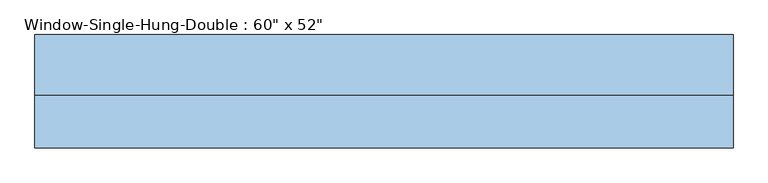
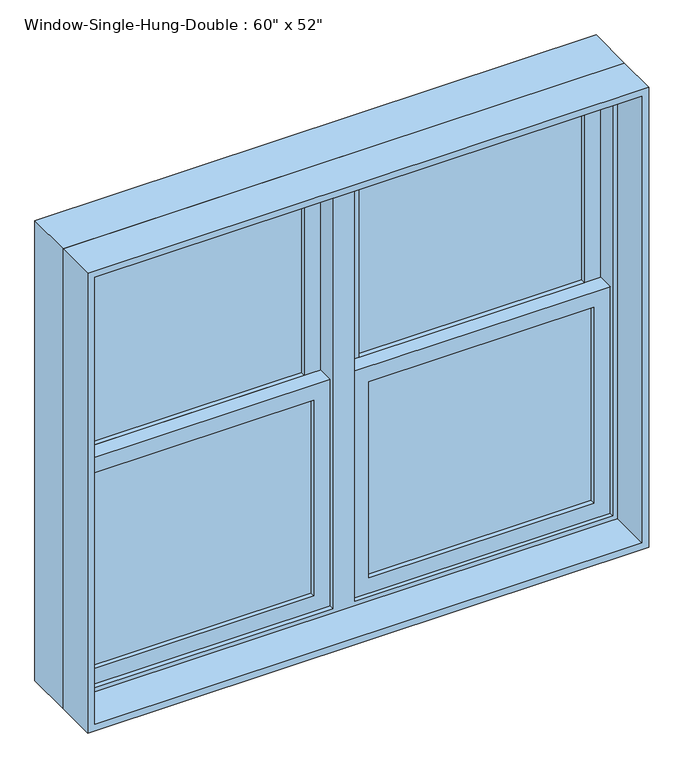
"""IFC4 building model written with IfcOpenShell, lengths in millimetres: window geometry."""

from ifc_helpers import new_model, si_unit, frame, origin, place, context, project, spatial, polyline, outline, extrude, source, transform, mapped, element, save


def window_bf3e2632(model_context):
    return source(origin(), model_context, "Body", "SweptSolid", [
        extrude(outline(polyline([(2235.2, 762.0), (2235.2, -762.0), (914.4, -762.0), (914.4, 762.0), (2235.2, 762.0)]), holes=[polyline([(2216.15, 742.95), (933.45, 742.95), (933.45, -742.95), (2216.15, -742.95), (2216.15, 742.95)])]), frame((0.0, -114.3, 0.0), z_axis=(0.0, 1.0, 0.0), x_axis=(0.0, 0.0, 1.0)), (0.0, 0.0, 1.0), 114.3),
        extrude(outline(polyline([(2203.45, 30.1625), (1552.575, 30.1625), (1552.575, 730.25), (2203.45, 730.25), (2203.45, 30.1625)]), holes=[polyline([(2159.0, 685.8), (1597.025, 685.8), (1597.025, 74.6125), (2159.0, 74.6125), (2159.0, 685.8)])]), frame((0.0, 57.15, 0.0), z_axis=(0.0, 1.0, 0.0), x_axis=(0.0, 0.0, 1.0)), (0.0, 0.0, 1.0), 44.45),
        extrude(outline(polyline([(1597.025, 30.1625), (946.15, 30.1625), (946.15, 730.25), (1597.025, 730.25), (1597.025, 30.1625)]), holes=[polyline([(1552.575, 685.8), (990.6, 685.8), (990.6, 74.6125), (1552.575, 74.6125), (1552.575, 685.8)])]), frame((0.0, 12.7, 0.0), z_axis=(0.0, 1.0, 0.0), x_axis=(0.0, 0.0, 1.0)), (0.0, 0.0, 1.0), 44.45),
        extrude(outline(polyline([(685.8, 88.9), (685.8, 82.55), (74.6125, 82.55), (74.6125, 88.9), (685.8, 88.9)])), frame((0.0, 0.0, 1597.025), z_axis=(0.0, 0.0, 1.0), x_axis=(1.0, 0.0, 0.0)), (0.0, 0.0, 1.0), 561.975),
        extrude(outline(polyline([(74.6125, 76.2), (685.8, 76.2), (685.8, 69.85), (74.6125, 69.85), (74.6125, 76.2)])), frame((0.0, 0.0, 1597.025), z_axis=(0.0, 0.0, 1.0), x_axis=(1.0, 0.0, 0.0)), (0.0, 0.0, 1.0), 561.975),
        extrude(outline(polyline([(685.8, 44.45), (685.8, 38.1), (74.6125, 38.1), (74.6125, 44.45), (685.8, 44.45)])), frame((0.0, 0.0, 990.6), z_axis=(0.0, 0.0, 1.0), x_axis=(1.0, 0.0, 0.0)), (0.0, 0.0, 1.0), 561.975),
        extrude(outline(polyline([(74.6125, 31.75), (685.8, 31.75), (685.8, 25.4), (74.6125, 25.4), (74.6125, 31.75)])), frame((0.0, 0.0, 990.6), z_axis=(0.0, 0.0, 1.0), x_axis=(1.0, 0.0, 0.0)), (0.0, 0.0, 1.0), 561.975),
        extrude(outline(polyline([(2203.45, -730.25), (1552.575, -730.25), (1552.575, -30.1625), (2203.45, -30.1625), (2203.45, -730.25)]), holes=[polyline([(2159.0, -74.6125), (1597.025, -74.6125), (1597.025, -685.8), (2159.0, -685.8), (2159.0, -74.6125)])]), frame((0.0, 57.15, 0.0), z_axis=(0.0, 1.0, 0.0), x_axis=(0.0, 0.0, 1.0)), (0.0, 0.0, 1.0), 44.45),
        extrude(outline(polyline([(1597.025, -730.25), (946.15, -730.25), (946.15, -30.1625), (1597.025, -30.1625), (1597.025, -730.25)]), holes=[polyline([(1552.575, -74.6125), (990.6, -74.6125), (990.6, -685.8), (1552.575, -685.8), (1552.575, -74.6125)])]), frame((0.0, 12.7, 0.0), z_axis=(0.0, 1.0, 0.0), x_axis=(0.0, 0.0, 1.0)), (0.0, 0.0, 1.0), 44.45),
        extrude(outline(polyline([(-685.8, 88.9), (-74.6125, 88.9), (-74.6125, 82.55), (-685.8, 82.55), (-685.8, 88.9)])), frame((0.0, 0.0, 1597.025), z_axis=(0.0, 0.0, 1.0), x_axis=(1.0, 0.0, 0.0)), (0.0, 0.0, 1.0), 561.975),
        extrude(outline(polyline([(-74.6125, 76.2), (-74.6125, 69.85), (-685.8, 69.85), (-685.8, 76.2), (-74.6125, 76.2)])), frame((0.0, 0.0, 1597.025), z_axis=(0.0, 0.0, 1.0), x_axis=(1.0, 0.0, 0.0)), (0.0, 0.0, 1.0), 561.975),
        extrude(outline(polyline([(-685.8, 44.45), (-74.6125, 44.45), (-74.6125, 38.1), (-685.8, 38.1), (-685.8, 44.45)])), frame((0.0, 0.0, 990.6), z_axis=(0.0, 0.0, 1.0), x_axis=(1.0, 0.0, 0.0)), (0.0, 0.0, 1.0), 561.975),
        extrude(outline(polyline([(-74.6125, 31.75), (-74.6125, 25.4), (-685.8, 25.4), (-685.8, 31.75), (-74.6125, 31.75)])), frame((0.0, 0.0, 990.6), z_axis=(0.0, 0.0, 1.0), x_axis=(1.0, 0.0, 0.0)), (0.0, 0.0, 1.0), 561.975),
        extrude(outline(polyline([(2235.2, 762.0), (2235.2, -762.0), (914.4, -762.0), (914.4, 762.0), (2235.2, 762.0)]), holes=[polyline([(946.15, -730.25), (2203.45, -730.25), (2203.45, -30.1625), (946.15, -30.1625), (946.15, -730.25)]), polyline([(946.15, 730.25), (946.15, 30.1625), (2203.45, 30.1625), (2203.45, 730.25), (946.15, 730.25)])]), frame((0.0, 0.0, 0.0), z_axis=(0.0, 1.0, 0.0), x_axis=(0.0, 0.0, 1.0)), (0.0, 0.0, 1.0), 133.35),
    ])


if __name__ == "__main__":
    model = new_model("IFC4")
    model_context = context("Model", 3, world=origin())
    ifc_project = project(units=[si_unit("LENGTHUNIT", "METRE", prefix="MILLI")], contexts=[model_context])
    site = spatial("IfcSite", under=ifc_project)
    building = spatial("IfcBuilding", under=site)
    placement = place(None, origin())
    window_shape = window_bf3e2632(model_context)
    element("IfcWindow", 1, ObjectType="Window-Single-Hung-Double : 60\" x 52\"", at=placement, inside=building, context=model_context, shape_type="MappedRepresentation", body=[
        mapped(window_shape, transform((0.0, 0.0, 0.0), x_axis=(1.0, 0.0, 0.0), y_axis=(0.0, 1.0, 0.0), z_axis=(0.0, 0.0, 1.0))),
    ])
    save(model, "model.ifc")

# Revit data of these elements
# Type "Window-Single-Hung-Double : 60\" x 52\""
#   Type Mark = "18"
#   Fire Rating = "0.5h"
#   Construction Type Id = "DG-DR"
#   Analytic Construction = "Double glazing - domestic"
#   Wall Thickness [instance default] = 0' - 6"
#   Window Inset [instance default] = 0' - 0"
#   Visual Light Transmittance = 0.81
#   Thermal Resistance (R) = 1.8146 (h·ft²·°F)/BTU
#   Solar Heat Gain Coefficient = 0.76
#   Muntin Width = 2' - 0 1/16"
#   Muntin Height = 1' - 10 1/8"
#   Interior Wall Closure [instance default] = 0' - 1 1/2"
#   Rough Width = 5' - 0 1/2"
#   Rough Height = 4' - 4 1/2"
#   Frame Extension [instance default] = 0' - 1 1/4"
#   Exterior Wall Closure [instance default] = 0' - 0 1/2"
#   Extension Jamb [instance default] = 0' - 1 1/2"
#   Heat Transfer Coefficient (U) = 0.5511 BTU/(h·ft²·°F)
#   Height = 4' - 4"
#   Width = 5' - 0"
#   Top Muntin Visibility = yes
#   Indicator Visibility [instance default] = yes
#   Extension Jamb Visibility [instance default] = yes
#   Interior Trim Visibility [instance default] = yes
#   Exterior Trim Visibility [instance default] = yes
#   Define Thermal Properties by = 1
#   Bottom Muntin Visibility = yes
#   Muntin Pattern = Muntin Pattern_2x2 : Muntin Pattern_2x2
#   Interior Trim = Trim-Window-Interior-Flat : Picture Frame
#   Interior Trim Material = Wood - Stained
#   Exterior Trim Material = Clad - White
#   Exterior Trim = Trim-Window-Exterior-Flat : with Sill
#   Glass Panel Material = Glass
#   Exterior Frame Material = Clad - White
#   Interior Frame Material = Wood - Stained
#   Wall Closure = (empty or 0)
# Element 1 (IfcWindow, "Window-Single-Hung-Double : 60\" x 52\"")
#   Wall Thickness = 0' - 9"
#   Extension Jamb = 0' - 4 1/2"
#   Materials on its faces: "Wood - Stained", "Glass", "Clad - White"
# Materials
#   "Wood - Stained": class "Wood", colour RGB 224 178 126, transparency 0, Cost = 0
#   "Clad - White": class "Wood", colour RGB 242 242 238, transparency 0, Cost = 0
#   "Glass": class "Glass", colour RGB 0 128 192, transparency 0.75, Description = "Soda Lime Glass", Cost = 0
